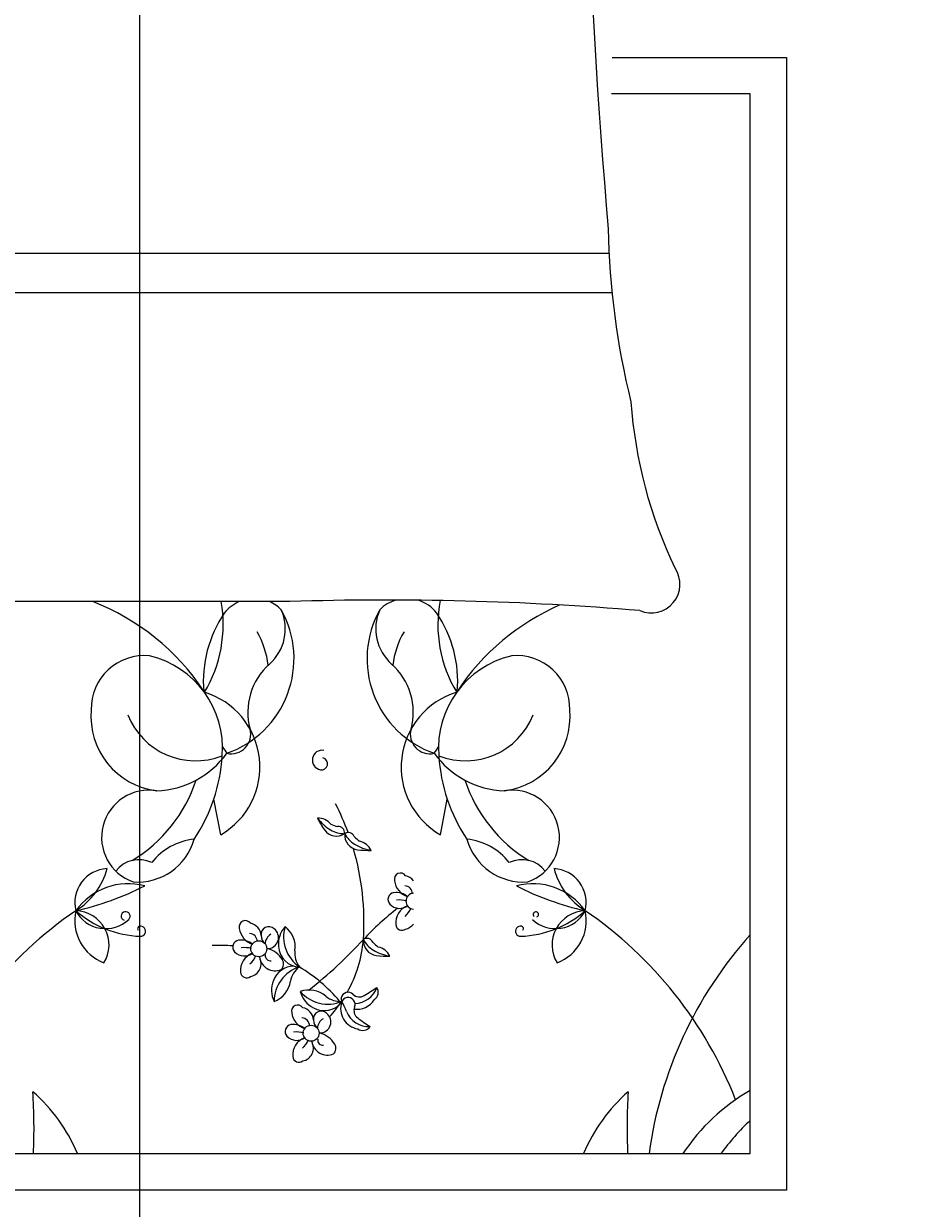
# Model space of a CAD drawing. Units: inches. Extents: x 0 to 281, y -535 to 46.
# Tile 17 of 22: x 112 to 134, y -66 to -36. Entities that reach past the tile are written whole.
import ezdxf

# ---------------------------------------------------------------- set-up
doc = ezdxf.new("R2010")
doc.units = ezdxf.units.IN
doc.header["$MEASUREMENT"] = 0
doc.layers.add('A-ANNO-DIMS', color=2, linetype='Continuous', lineweight=18)
doc.layers.add('A-FURN', color=8, linetype='Continuous', lineweight=18)
doc.styles.get("Standard").update_dxf_attribs({"font": 'arial.ttf'})
doc.dimstyles.get("Standard").update_dxf_attribs({"dimtxt": 0.18, "dimasz": 0.18, "dimexe": 0.18, "dimexo": 0.0625, "dimgap": 0.09, "dimtad": 0, "dimtih": 1, "dimtoh": 1, "dimdec": 0, "dimzin": 0, "dimdsep": 46, "dimlunit": 3, "dimtxsty": 'Standard', "dimcen": 0.09, "dimadec": 0, "dimazin": 0, "dimtfac": 1, "dimtdec": 0, "dimtofl": 0, "dimtmove": 0, "dimatfit": 3, "dimfxl": 1, "dimtolj": 1, "dimtzin": 0, "dimarcsym": 0})

# ---------------------------------------------------------------- blocks, each defined once
blk = doc.blocks.new('*D45')
at = {"layer": 'A-ANNO-DIMS', "color": 0, "lineweight": -2, "transparency": 16777216}
for p, q in [((114.459, -263.348), (114.459, 46.219)), ((114.639, 46.039), (132.13, 46.039)), ((150.279, 46.039), (132.788, 46.039)), ((150.459, -263.348), (150.459, 46.219))]:
    blk.add_line(p, q, dxfattribs=at)
at = {"layer": 'A-ANNO-DIMS', "color": 0, "transparency": 16777216}
for points in [[(114.639, 46.069), (114.639, 46.009), (114.459, 46.039)], [(150.279, 46.069), (150.279, 46.009), (150.459, 46.039)]]:
    blk.add_solid(points, dxfattribs=at)
at = {"layer": 'Defpoints', "color": 0, "transparency": 16777216}
for p in [(150.459, 46.039), (114.459, -263.411), (150.459, -263.411)]:
    blk.add_point(p, dxfattribs=at)
at = {"layer": 'A-ANNO-DIMS', "color": 0, "transparency": 16777216, "insert": (132.459, 46.039), "char_height": 0.18, "attachment_point": 5}
blk.add_mtext('\\A1;3\'-0"', dxfattribs=at)
blk = doc.blocks.new('*D47')
at = {"layer": 'A-ANNO-DIMS', "color": 0, "lineweight": -2, "transparency": 16777216}
for p, q in [((114.459, -392.348), (114.459, 46.219)), ((114.639, 46.039), (132.13, 46.039)), ((150.279, 46.039), (132.788, 46.039)), ((150.459, -392.348), (150.459, 46.219))]:
    blk.add_line(p, q, dxfattribs=at)
at = {"layer": 'A-ANNO-DIMS', "color": 0, "transparency": 16777216}
for points in [[(114.639, 46.069), (114.639, 46.009), (114.459, 46.039)], [(150.279, 46.069), (150.279, 46.009), (150.459, 46.039)]]:
    blk.add_solid(points, dxfattribs=at)
at = {"layer": 'Defpoints', "color": 0, "transparency": 16777216}
for p in [(150.459, 46.039), (114.459, -392.411), (150.459, -392.411)]:
    blk.add_point(p, dxfattribs=at)
at = {"layer": 'A-ANNO-DIMS', "color": 0, "transparency": 16777216, "insert": (132.459, 46.039), "char_height": 0.18, "attachment_point": 5}
blk.add_mtext('\\A1;3\'-0"', dxfattribs=at)

msp = doc.modelspace()

# ---------------------------------------------------------------- linework, layer by layer
at = {"layer": 'A-FURN'}
for p, q in [((126.362, -37.076), (130.754, -37.076)), ((130.754, -37.076), (130.754, -65.604)), ((129.836, -37.994), (126.345, -37.994)), ((129.836, -64.686), (129.836, -37.994)), ((126.28, -42.015), (77.493, -42.015)), ((126.355, -43.003), (77.492, -43.003)), ((118.239, -50.782), (86.086, -50.782)), ((116.497, -56.657), (116.322, -55.762)), ((122.032, -56.657), (122.207, -55.762)), ((73.937, -64.686), (129.836, -64.686)), ((130.754, -65.604), (73.019, -65.604))]:
    msp.add_line(p, q, dxfattribs=at)
msp.add_lwpolyline([(126.258, -41.392, 0.056112), (126.833, -45.749, 0.095341), (127.946, -49.946)], format="xyb", dxfattribs=at)
for centre in [(117.457, -59.527), (118.776, -61.653)]:
    msp.add_circle(centre, 0.202, dxfattribs=at)
for centre, radius, start, end in [((311.205, -25.622), 185.618, 179.11454, 184.87351), ((127.346, -50.347), 0.722, 246.5219, 33.8264), ((111.082, -56.359), 5.994, 33.6671, 68.5059), ((113.28, -51.368), 3.281, 328.8218, 10.2867), ((117.344, -51.658), 0.954, 113.2856, 142.325), ((115.821, -52.22), 2.524, 289.2822, 29.1751), ((117.344, -51.658), 0.954, 44.4517, 66.7144), ((116.941, -51.469), 1.185, 311.5653, 23.8354), ((120.665, -127.804), 77.06, 85.24024, 91.80351), ((122.708, -52.22), 2.524, 150.8249, 250.7178), ((121.589, -51.469), 1.185, 156.1646, 228.4347), ((121.186, -51.658), 0.954, 106.6343, 135.5483), ((121.186, -51.658), 0.954, 37.675, 72.5814), ((125.25, -51.368), 3.281, 169.249, 211.1782), ((127.448, -56.359), 5.994, 113.6453, 146.3329), ((119.114, -52.792), 3.054, 145.785, 184.7304), ((119.415, -52.792), 3.054, 355.2696, 34.215), ((115.44, -52.677), 2.276, 7.436, 29.9149), ((123.089, -52.677), 2.276, 150.0851, 172.564), ((114.573, -53.481), 1.337, 84.4856, 181.0538), ((114.163, -54.47), 2.382, 355.2933, 76.921), ((124.367, -54.47), 2.382, 103.079, 184.7067), ((123.956, -53.481), 1.337, 358.9462, 95.5144), ((118.804, -53.57), 1.624, 131.5653, 195.1471), ((119.725, -53.57), 1.624, 344.8529, 48.4347), ((115.516, -54.95), 1.969, 299.9085, 73.1337), ((123.014, -54.95), 1.969, 106.8663, 240.0915), ((115.121, -53.672), 1.892, 174.9449, 262.8857), ((115.865, -52.955), 1.838, 201.5819, 291.4221), ((122.664, -52.955), 1.838, 248.5779, 338.4181), ((123.408, -53.672), 1.892, 277.1143, 5.0551), ((116.762, -54.123), 0.492, 257.3041, 15.1471), ((121.767, -54.123), 0.492, 164.8529, 282.6959), ((119.114, -52.792), 3.054, 212.7011, 216.3445), ((119.055, -54.775), 0.248, 79.5864, 259.5616), ((119.415, -52.792), 3.054, 323.6555, 327.2989), ((114.792, -53.252), 2.3, 272.3591, 324.0401), ((112.295, -54.407), 4.25, 326.2883, 356.5076), ((119.037, -54.869), 0.153, 259.5616, 77.2949), ((123.737, -53.252), 2.3, 215.9599, 267.6409), ((126.235, -54.407), 4.25, 183.4924, 213.7117), ((112.33, -54.105), 3.739, 301.2614, 341.7045), ((126.2, -54.105), 3.739, 198.2955, 238.7386), ((114.686, -56.721), 1.188, 80.264, 250.8688), ((123.843, -56.721), 1.188, 289.1312, 99.736), ((113.548, -58.855), 6.559, 20.1059, 26.9968), ((119.916, -55.461), 1.252, 218.4388, 238.836), ((118.954, -56.655), 0.416, 39.5056, 92.6421), ((120.934, -55.242), 2.233, 206.5064, 215.3102), ((119.417, -56.307), 0.38, 216.5232, 302.4668), ((119.611, -55.964), 0.664, 238.836, 270.8141), ((119.785, -55.224), 1.272, 246.3901, 254.4871), ((119.46, -56.611), 0.161, 353.9457, 95.6216), ((120, -56.656), 0.38, 175.7131, 261.6568), ((119.712, -56.761), 0.161, 22.5583, 124.2343), ((120.21, -56.323), 0.664, 207.3659, 239.344), ((114.401, -56.364), 1.484, 265.969, 344.3045), ((115.999, -58.337), 1.581, 96.1662, 141.5825), ((120.781, -55.82), 1.272, 223.6929, 231.7899), ((120.51, -55.817), 1.252, 239.344, 259.7412), ((119.912, -57.228), 0.416, 25.5379, 78.6744), ((124.129, -56.364), 1.484, 195.6955, 274.031), ((122.53, -58.337), 1.581, 38.4175, 83.8338), ((114.441, -58.009), 0.728, 63.9755, 143.2681), ((113.548, -58.855), 6.559, 356.1723, 16.4158), ((120.222, -54.816), 2.233, 262.8698, 271.6736), ((124.088, -58.009), 0.728, 36.7319, 116.0245), ((113.679, -58.364), 0.857, 92.9516, 193.728), ((111.927, -57.06), 1.766, 301.3827, 345.2969), ((126.603, -57.06), 1.766, 194.7031, 238.6173), ((124.85, -58.364), 0.857, 346.272, 87.0484), ((121.028, -57.776), 0.156, 35.0752, 194.7644), ((121.358, -57.752), 0.485, 187.4968, 251.2737), ((121.088, -58.016), 0.336, 37.3642, 78.4363), ((114.173, -59.523), 1.635, 75.4653, 144.2343), ((111.278, -51.505), 7.235, 282.5173, 297.1824), ((120.886, -58.285), 0.174, 99.6513, 222.3208), ((120.927, -58.525), 0.417, 46.3462, 99.6513), ((121.132, -58.137), 0.193, 358.1325, 88.8919), ((121.367, -58.328), 0.202, 93.2768, 266.7232), ((124.356, -59.523), 1.635, 35.7657, 104.5347), ((127.251, -51.505), 7.235, 242.8176, 257.4827), ((121.002, -58.18), 0.33, 222.3208, 310.2111), ((121.374, -58.879), 0.469, 111.6382, 184.947), ((121.006, -58.958), 0.66, 74.2829, 96.9148), ((118.687, -67.102), 10.341, 124.3865, 158.5908), ((113.967, -58.812), 1.147, 167.7115, 249.0387), ((113.596, -58.175), 0.846, 207.6827, 313.7762), ((114.568, -56.599), 2.615, 228.8402, 267.9352), ((112.821, -59.431), 0.864, 328.4633, 88.2869), ((114.103, -58.705), 0.112, 313.7762, 249.7183), ((125.578, -64.435), 7.519, 127.9541, 136.8459), ((120.732, -58.258), 0.612, 312.3896, 336.5724), ((123.962, -56.599), 2.615, 272.0648, 311.1598), ((124.934, -58.175), 0.846, 226.2238, 332.3173), ((124.438, -58.662), 0.0674, 290.2667, 226.2271), ((125.709, -59.431), 0.864, 91.7131, 211.5367), ((124.562, -58.812), 1.147, 290.9613, 12.2885), ((119.842, -67.102), 10.341, 21.4092, 55.6135), ((114.465, -59.019), 0.0624, 101.4834, 217.9409), ((114.478, -59.084), 0.128, 267.9352, 101.4834), ((117.118, -58.974), 0.156, 35.0752, 194.7644), ((117.448, -58.951), 0.485, 187.4968, 251.2737), ((117.178, -59.214), 0.336, 3.635, 78.4363), ((117.71, -59.171), 0.198, 48.2946, 186.2474), ((117.679, -59.246), 0.275, 268.5719, 53.8954), ((118.618, -59.412), 0.668, 138.342, 184.9894), ((119.001, -59.227), 0.919, 163.6301, 235.4631), ((117.725, -59.485), 0.65, 352.0748, 52.6895), ((121.061, -58.906), 0.155, 184.947, 307.5263), ((121.092, -58.702), 0.333, 280.9597, 322.2379), ((124.051, -59.084), 0.128, 78.5166, 272.0648), ((124.064, -59.019), 0.0624, 322.0591, 78.5166), ((116.976, -59.484), 0.174, 99.6513, 222.3208), ((117.017, -59.723), 0.417, 46.3462, 99.6513), ((117.222, -59.336), 0.193, 358.1325, 88.8919), ((117.83, -59.17), 0.317, 184.2123, 228.1587), ((117.896, -59.406), 0.278, 118.8493, 179.9355), ((112.082, -52.018), 10.821, 307.8256, 317.7588), ((116.816, -59.02), 3.288, 330.7959, 355.244), ((120.472, -59.321), 0.38, 175.7131, 261.6568), ((120.183, -59.426), 0.161, 22.5583, 124.2343), ((120.682, -58.987), 0.664, 207.3659, 239.344), ((121.252, -58.485), 1.272, 223.6929, 231.7899), ((137.535, -66.079), 10.341, 138.1144, 172.255), ((116.478, -63.387), 3.944, 85.2415, 92.8929), ((117.092, -59.378), 0.33, 222.3208, 310.2111), ((117.464, -60.077), 0.469, 111.6382, 184.947), ((117.096, -60.157), 0.66, 74.2829, 96.9148), ((117.511, -60.136), 0.636, 31.9501, 75.2442), ((118.51, -59.432), 0.559, 183.8774, 267.1501), ((118.904, -59.649), 0.541, 172.0748, 218.2393), ((120.982, -58.482), 1.252, 239.344, 259.7412), ((120.384, -59.892), 0.416, 25.5379, 78.6744), ((116.823, -59.457), 0.612, 312.3896, 336.5724), ((117.182, -59.9), 0.333, 280.9597, 28.7804), ((117.867, -59.681), 0.398, 188.5614, 292.5914), ((117.755, -59.697), 0.134, 172.868, 277.094), ((118.35, -60.522), 0.559, 91.4625, 159.4747), ((117.881, -59.905), 0.2, 314.3732, 31.9501), ((116.478, -63.387), 3.944, 66.1523, 66.9499), ((120.694, -57.481), 2.233, 262.8698, 271.6736), ((117.151, -60.104), 0.155, 184.947, 307.5263), ((118.762, -60.859), 0.919, 107.889, 179.722), ((118.791, -60.427), 0.541, 125.1128, 171.2773), ((116.478, -63.387), 3.944, 40.182, 59.456), ((118.448, -60.572), 0.668, 158.3627, 205.0101), ((117.613, -60.246), 0.65, 290.6625, 351.2773), ((119.857, -60.295), 0.61, 272.3172, 340.5201), ((117.068, -55.661), 5.892, 301.1156, 304.8118), ((120.243, -60.622), 0.225, 303.0979, 33.1364), ((118.724, -61.216), 0.65, 49.3812, 109.9959), ((119.196, -60.002), 0.919, 220.9365, 292.7695), ((119.145, -60.424), 0.668, 195.6484, 242.2957), ((119.5, -60.311), 0.541, 229.3812, 275.5456), ((116.816, -59.02), 3.288, 317.5083, 325.9967), ((119.707, -60.799), 0.176, 45.7354, 228.1297), ((119.708, -60.931), 0.176, 338.2452, 160.6395), ((116.401, -62.402), 3.513, 21.7087, 26.2181), ((119.993, -60.506), 0.233, 225.7354, 301.1156), ((119.925, -60.526), 0.525, 262.6008, 327.1845), ((118.437, -61.1), 0.156, 35.0752, 194.7644), ((118.767, -61.077), 0.485, 187.4968, 251.2737), ((118.497, -61.34), 0.336, 3.635, 78.4363), ((119.029, -61.297), 0.198, 48.2946, 186.2474), ((119.104, -60.526), 0.559, 241.1838, 321.6792), ((118.999, -61.372), 0.275, 268.5719, 53.8954), ((120.044, -61.028), 0.525, 162.8042, 259.6943), ((120.23, -60.877), 0.61, 201.7087, 273.0299), ((120.088, -61.082), 0.233, 158.2452, 233.6254), ((118.296, -61.609), 0.174, 99.6513, 222.3208), ((118.336, -61.849), 0.417, 46.3462, 99.6513), ((118.541, -61.462), 0.193, 358.1325, 88.8919), ((119.149, -61.296), 0.317, 184.2123, 228.1587), ((119.215, -61.532), 0.278, 118.8493, 179.9355), ((123.444, -56.526), 5.892, 233.6254, 237.3216), ((118.411, -61.504), 0.33, 222.3208, 310.2111), ((118.415, -62.282), 0.66, 74.2829, 96.9148), ((118.83, -62.262), 0.636, 31.9501, 75.2442), ((120.077, -61.359), 0.225, 235.6077, 325.6462), ((118.783, -62.203), 0.469, 111.6382, 184.947), ((118.142, -61.582), 0.612, 312.3896, 336.5724), ((118.501, -62.026), 0.333, 280.9597, 28.7804), ((119.187, -61.806), 0.398, 188.5614, 292.5914), ((119.075, -61.823), 0.134, 172.868, 277.094), ((119.2, -62.031), 0.2, 314.3732, 31.9501), ((118.47, -62.23), 0.155, 184.947, 307.5263), ((97.487, -64.039), 14.308, 357.4081, 3.6519), ((109.005, -66.299), 4.205, 22.5547, 48.9546), ((129.525, -66.299), 4.205, 131.0454, 157.4453), ((141.043, -64.039), 14.308, 176.3481, 182.5919), ((132.347, -67.464), 5.039, 119.8884, 146.5383), ((134.16, -68.404), 6.28, 133.5186, 143.6964)]:
    msp.add_arc(centre, radius, start, end, dxfattribs=at)

# ---------------------------------------------------------------- dimensions: what is measured, and where the dimension line sits
at = {"layer": 'A-ANNO-DIMS'}
for p1, p2, picture in [((114.459, -263.411), (150.459, -263.411), '*D45'), ((114.459, -392.411), (150.459, -392.411), '*D47')]:
    dim = msp.add_linear_dim(base=(150.459, 46.039), p1=p1, p2=p2, dimstyle='Standard', override={"dimdec": 1, "dimlfac": 1, "dimrnd": 0, "dimzin": 1, "dimdsep": 46, "dimlunit": 4, "dimfrac": 2}, dxfattribs=at)
    dim.commit()
    dim.dimension.update_dxf_attribs({"geometry": picture, "text_midpoint": (132.459, 46.039)})

doc.saveas('drawing.dxf')
